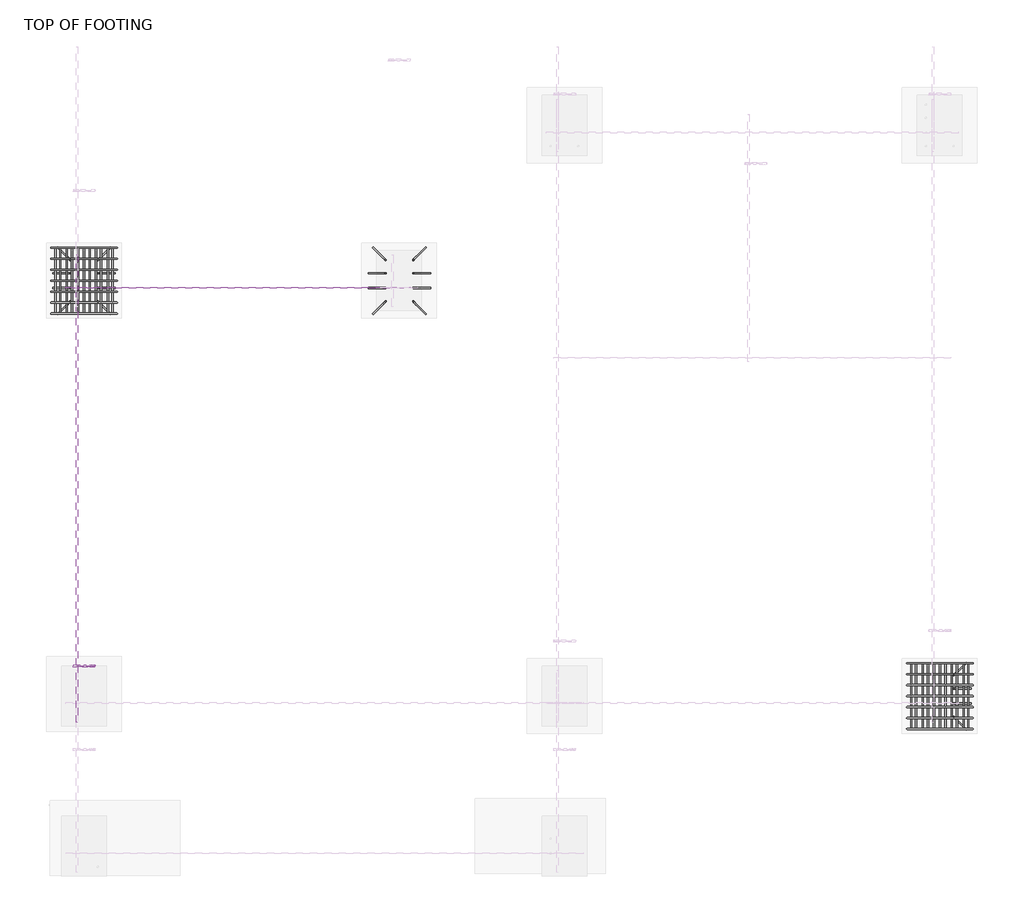
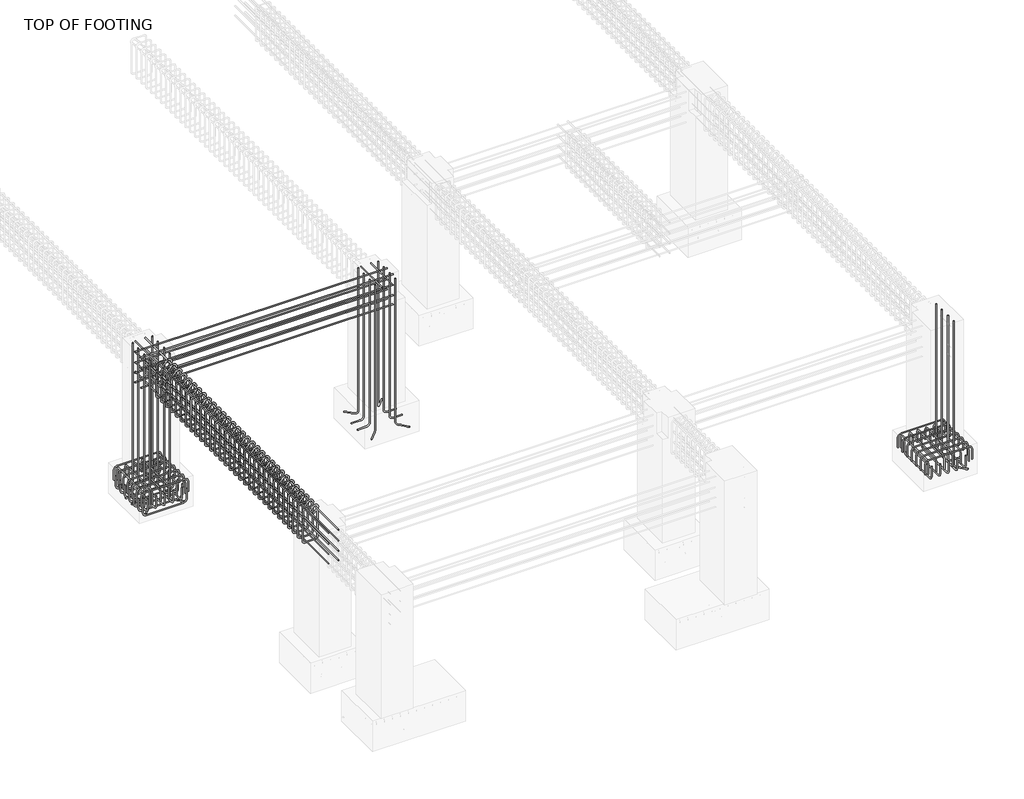
# One storey, part 4 of 8: 32 reinforcing bars.
"""IFC4 building model written with IfcOpenShell, lengths in millimetres."""

from ifc_helpers import new_model, si_unit, point, frame, origin, place, context, project, spatial, polyline, circle_curve, trimmed, segment, composite_curve, source, transform, mapped, element, save
from ifc_brep_helpers import swept_disk

model = new_model("IFC4")

# Units and contexts
model_context = context("Model", 3, world=origin())
ifc_project = project(units=[si_unit("LENGTHUNIT", "METRE", prefix="MILLI")], contexts=[model_context])

# Site, building, storey
site = spatial("IfcSite", under=ifc_project)
building = spatial("IfcBuilding", under=site)
storey = spatial("IfcBuildingStorey", under=building, Name="TOP OF FOOTING", Elevation=-1828.8)

# Reinforcing bars
placement = place(None, origin())
reinforcing_bar_shape = source(origin(), model_context, "Body", "SolidModel", [
    swept_disk(composite_curve([segment(polyline([(-6195.5877818, 3995.6420243, -2021.245224), (-6195.5877818, 3995.6420243, -2168.545224)]), True, "CONTINUOUS"), segment(trimmed(circle_curve(frame((-6241.9377818, 3995.6420243, -2168.545224), z_axis=(0.0, 1.0, 0.0), x_axis=(46.350000000000364, 0.0, 0.0)), 46.35), [point((-6195.5877818, 3995.6420243, -2168.545224))], [point((-6241.9377818, 3995.6420243, -2214.895224))], True, "CARTESIAN"), True, "CONTINUOUS"), segment(polyline([(-6241.9377818, 3995.6420243, -2214.895224), (-6762.8758647, 3995.6420243, -2214.895224)]), True, "CONTINUOUS"), segment(trimmed(circle_curve(frame((-6762.8758647, 3995.6420243, -2168.545224), z_axis=(0.0, 1.0, 0.0), x_axis=(0.0, 0.0, -46.34999999999991)), 46.35), [point((-6762.8758647, 3995.6420243, -2214.895224))], [point((-6809.2258647, 3995.6420243, -2168.545224))], True, "CARTESIAN"), True, "CONTINUOUS"), segment(polyline([(-6809.2258647, 3995.6420243, -2168.545224), (-6809.2258647, 3995.6420243, -2021.245224)]), True, "CONTINUOUS")], self_intersect=False), 6.35),
])
element("IfcReinforcingBar", 1, at=placement, inside=storey, context=model_context, shape_type="MappedRepresentation", body=[
    mapped(reinforcing_bar_shape, transform((0.0, 0.0, 0.0), x_axis=(1.0, 0.0, 0.0), y_axis=(0.0, 1.0, 0.0), z_axis=(0.0, 0.0, 1.0))),
    mapped(reinforcing_bar_shape, transform((0.0, -109.55, 0.0), x_axis=(1.0, 0.0, 0.0), y_axis=(0.0, 1.0, 0.0), z_axis=(0.0, 0.0, 1.0))),
    mapped(reinforcing_bar_shape, transform((0.0, -219.1, 0.0), x_axis=(1.0, 0.0, 0.0), y_axis=(0.0, 1.0, 0.0), z_axis=(0.0, 0.0, 1.0))),
    mapped(reinforcing_bar_shape, transform((0.0, -328.65, 0.0), x_axis=(1.0, 0.0, 0.0), y_axis=(0.0, 1.0, 0.0), z_axis=(0.0, 0.0, 1.0))),
    mapped(reinforcing_bar_shape, transform((0.0, -438.2, 0.0), x_axis=(1.0, 0.0, 0.0), y_axis=(0.0, 1.0, 0.0), z_axis=(0.0, 0.0, 1.0))),
    mapped(reinforcing_bar_shape, transform((0.0, -547.75, 0.0), x_axis=(1.0, 0.0, 0.0), y_axis=(0.0, 1.0, 0.0), z_axis=(0.0, 0.0, 1.0))),
    mapped(reinforcing_bar_shape, transform((0.0, -657.3, 0.0), x_axis=(1.0, 0.0, 0.0), y_axis=(0.0, 1.0, 0.0), z_axis=(0.0, 0.0, 1.0))),
])
reinforcing_bar_2_shape = source(origin(), model_context, "Body", "SolidModel", [
    swept_disk(composite_curve([segment(polyline([(-6831.1461367, 3995.6420243, -2068.8), (-6831.1461367, 3995.6420243, -1921.5)]), True, "CONTINUOUS"), segment(trimmed(circle_curve(frame((-6784.7961367, 3995.6420243, -1921.5), z_axis=(0.0, 1.0, 0.0), x_axis=(-46.350000000000364, 0.0, 0.0)), 46.35), [point((-6831.1461367, 3995.6420243, -1921.5))], [point((-6784.7961367, 3995.6420243, -1875.15))], True, "CARTESIAN"), True, "CONTINUOUS"), segment(polyline([(-6784.7961367, 3995.6420243, -1875.15), (-6220.1961367, 3995.6420243, -1875.15)]), True, "CONTINUOUS"), segment(trimmed(circle_curve(frame((-6220.1961367, 3995.6420243, -1921.5), z_axis=(0.0, 1.0, 0.0), x_axis=(0.0, 0.0, 46.34999999999991)), 46.35), [point((-6220.1961367, 3995.6420243, -1875.15))], [point((-6173.8461367, 3995.6420243, -1921.5))], True, "CARTESIAN"), True, "CONTINUOUS"), segment(polyline([(-6173.8461367, 3995.6420243, -1921.5), (-6173.8461367, 3995.6420243, -2068.8)]), True, "CONTINUOUS")], self_intersect=False), 6.35),
])
element("IfcReinforcingBar", 2, at=placement, inside=storey, context=model_context, shape_type="MappedRepresentation", body=[
    mapped(reinforcing_bar_2_shape, transform((0.0, 0.0, 0.0), x_axis=(1.0, 0.0, 0.0), y_axis=(0.0, 1.0, 0.0), z_axis=(0.0, 0.0, 1.0))),
    mapped(reinforcing_bar_2_shape, transform((0.0, -109.55, 0.0), x_axis=(1.0, 0.0, 0.0), y_axis=(0.0, 1.0, 0.0), z_axis=(0.0, 0.0, 1.0))),
    mapped(reinforcing_bar_2_shape, transform((0.0, -219.1, 0.0), x_axis=(1.0, 0.0, 0.0), y_axis=(0.0, 1.0, 0.0), z_axis=(0.0, 0.0, 1.0))),
    mapped(reinforcing_bar_2_shape, transform((0.0, -328.65, 0.0), x_axis=(1.0, 0.0, 0.0), y_axis=(0.0, 1.0, 0.0), z_axis=(0.0, 0.0, 1.0))),
    mapped(reinforcing_bar_2_shape, transform((0.0, -438.2, 0.0), x_axis=(1.0, 0.0, 0.0), y_axis=(0.0, 1.0, 0.0), z_axis=(0.0, 0.0, 1.0))),
    mapped(reinforcing_bar_2_shape, transform((0.0, -547.75, 0.0), x_axis=(1.0, 0.0, 0.0), y_axis=(0.0, 1.0, 0.0), z_axis=(0.0, 0.0, 1.0))),
    mapped(reinforcing_bar_2_shape, transform((0.0, -657.3, 0.0), x_axis=(1.0, 0.0, 0.0), y_axis=(0.0, 1.0, 0.0), z_axis=(0.0, 0.0, 1.0))),
])
reinforcing_bar_3_shape = source(origin(), model_context, "Body", "SolidModel", [
    swept_disk(composite_curve([segment(polyline([(-6219.0253093, 3995.6420243, -2080.9203068), (-6219.0253093, 3995.6420243, -1933.6203068)]), True, "CONTINUOUS"), segment(trimmed(circle_curve(frame((-6219.0253093, 3949.2920243, -1933.6203068), z_axis=(1.0, 0.0, 0.0), x_axis=(0.0, 46.34999999999991, 0.0)), 46.35), [point((-6219.0253093, 3995.6420243, -1933.6203068))], [point((-6219.0253093, 3949.2920243, -1887.2703068))], True, "CARTESIAN"), True, "CONTINUOUS"), segment(polyline([(-6219.0253093, 3949.2920243, -1887.2703068), (-6219.0253093, 3384.6920243, -1887.2703068)]), True, "CONTINUOUS"), segment(trimmed(circle_curve(frame((-6219.0253093, 3384.6920243, -1933.6203068), z_axis=(1.0, 0.0, 0.0), x_axis=(0.0, 0.0, 46.34999999999991)), 46.35), [point((-6219.0253093, 3384.6920243, -1887.2703068))], [point((-6219.0253093, 3338.3420243, -1933.6203068))], True, "CARTESIAN"), True, "CONTINUOUS"), segment(polyline([(-6219.0253093, 3338.3420243, -1933.6203068), (-6219.0253093, 3338.3420243, -2080.9203068)]), True, "CONTINUOUS")], self_intersect=False), 6.35),
])
element("IfcReinforcingBar", 3, at=placement, inside=storey, context=model_context, shape_type="MappedRepresentation", body=[
    mapped(reinforcing_bar_3_shape, transform((0.0, 0.0, 0.0), x_axis=(1.0, 0.0, 0.0), y_axis=(0.0, 1.0, 0.0), z_axis=(0.0, 0.0, 1.0))),
    mapped(reinforcing_bar_3_shape, transform((-113.9683653, 0.0, 0.0), x_axis=(1.0, 0.0, 0.0), y_axis=(0.0, 1.0, 0.0), z_axis=(0.0, 0.0, 1.0))),
    mapped(reinforcing_bar_3_shape, transform((-227.9367307, 0.0, 0.0), x_axis=(1.0, 0.0, 0.0), y_axis=(0.0, 1.0, 0.0), z_axis=(0.0, 0.0, 1.0))),
    mapped(reinforcing_bar_3_shape, transform((-341.905096, 0.0, 0.0), x_axis=(1.0, 0.0, 0.0), y_axis=(0.0, 1.0, 0.0), z_axis=(0.0, 0.0, 1.0))),
    mapped(reinforcing_bar_3_shape, transform((-455.8734613, 0.0, 0.0), x_axis=(1.0, 0.0, 0.0), y_axis=(0.0, 1.0, 0.0), z_axis=(0.0, 0.0, 1.0))),
    mapped(reinforcing_bar_3_shape, transform((-569.8418267, 0.0, 0.0), x_axis=(1.0, 0.0, 0.0), y_axis=(0.0, 1.0, 0.0), z_axis=(0.0, 0.0, 1.0))),
])
reinforcing_bar_4_shape = source(origin(), model_context, "Body", "SolidModel", [
    swept_disk(composite_curve([segment(polyline([(-6741.3656272, 3995.6420243, -1984.9681267), (-6741.3656272, 3995.6420243, -2132.2681267)]), True, "CONTINUOUS"), segment(trimmed(circle_curve(frame((-6741.3656272, 3949.2920243, -2132.2681267), z_axis=(-1.0, 0.0, 0.0), x_axis=(0.0, 46.34999999999991, 0.0)), 46.35), [point((-6741.3656272, 3995.6420243, -2132.2681267))], [point((-6741.3656272, 3949.2920243, -2178.6181267))], True, "CARTESIAN"), True, "CONTINUOUS"), segment(polyline([(-6741.3656272, 3949.2920243, -2178.6181267), (-6741.3656272, 3384.6920243, -2178.6181267)]), True, "CONTINUOUS"), segment(trimmed(circle_curve(frame((-6741.3656272, 3384.6920243, -2132.2681267), z_axis=(-1.0, 0.0, 0.0), x_axis=(0.0, 0.0, -46.350000000000364)), 46.35), [point((-6741.3656272, 3384.6920243, -2178.6181267))], [point((-6741.3656272, 3338.3420243, -2132.2681267))], True, "CARTESIAN"), True, "CONTINUOUS"), segment(polyline([(-6741.3656272, 3338.3420243, -2132.2681267), (-6741.3656272, 3338.3420243, -1984.9681267)]), True, "CONTINUOUS")], self_intersect=False), 6.35),
])
element("IfcReinforcingBar", 4, at=placement, inside=storey, context=model_context, shape_type="MappedRepresentation", body=[
    mapped(reinforcing_bar_4_shape, transform((0.0, 0.0, 0.0), x_axis=(1.0, 0.0, 0.0), y_axis=(0.0, 1.0, 0.0), z_axis=(0.0, 0.0, 1.0))),
    mapped(reinforcing_bar_4_shape, transform((119.2770606, 0.0, 0.0), x_axis=(1.0, 0.0, 0.0), y_axis=(0.0, 1.0, 0.0), z_axis=(0.0, 0.0, 1.0))),
    mapped(reinforcing_bar_4_shape, transform((238.5541211, 0.0, 0.0), x_axis=(1.0, 0.0, 0.0), y_axis=(0.0, 1.0, 0.0), z_axis=(0.0, 0.0, 1.0))),
    mapped(reinforcing_bar_4_shape, transform((357.8311817, 0.0, 0.0), x_axis=(1.0, 0.0, 0.0), y_axis=(0.0, 1.0, 0.0), z_axis=(0.0, 0.0, 1.0))),
    mapped(reinforcing_bar_4_shape, transform((477.1082423, 0.0, 0.0), x_axis=(1.0, 0.0, 0.0), y_axis=(0.0, 1.0, 0.0), z_axis=(0.0, 0.0, 1.0))),
])
reinforcing_bar_5_shape = source(origin(), model_context, "Body", "SolidModel", [
    swept_disk(composite_curve([segment(polyline([(1718.8538633, -154.3579757, -2068.8), (1718.8538633, -154.3579757, -1921.5)]), True, "CONTINUOUS"), segment(trimmed(circle_curve(frame((1765.2038633, -154.3579757, -1921.5), z_axis=(0.0, 1.0, 0.0), x_axis=(-46.34999999999991, 0.0, 0.0)), 46.35), [point((1718.8538633, -154.3579757, -1921.5))], [point((1765.2038633, -154.3579757, -1875.15))], True, "CARTESIAN"), True, "CONTINUOUS"), segment(polyline([(1765.2038633, -154.3579757, -1875.15), (2329.8038633, -154.3579757, -1875.15)]), True, "CONTINUOUS"), segment(trimmed(circle_curve(frame((2329.8038633, -154.3579757, -1921.5), z_axis=(0.0, 1.0, 0.0), x_axis=(0.0, 0.0, 46.34999999999991)), 46.35), [point((2329.8038633, -154.3579757, -1875.15))], [point((2376.1538633, -154.3579757, -1921.5))], True, "CARTESIAN"), True, "CONTINUOUS"), segment(polyline([(2376.1538633, -154.3579757, -1921.5), (2376.1538633, -154.3579757, -2068.8)]), True, "CONTINUOUS")], self_intersect=False), 6.35),
])
element("IfcReinforcingBar", 5, at=placement, inside=storey, context=model_context, shape_type="MappedRepresentation", body=[
    mapped(reinforcing_bar_5_shape, transform((0.0, 0.0, 0.0), x_axis=(1.0, 0.0, 0.0), y_axis=(0.0, 1.0, 0.0), z_axis=(0.0, 0.0, 1.0))),
    mapped(reinforcing_bar_5_shape, transform((0.0, -109.55, 0.0), x_axis=(1.0, 0.0, 0.0), y_axis=(0.0, 1.0, 0.0), z_axis=(0.0, 0.0, 1.0))),
    mapped(reinforcing_bar_5_shape, transform((0.0, -219.1, 0.0), x_axis=(1.0, 0.0, 0.0), y_axis=(0.0, 1.0, 0.0), z_axis=(0.0, 0.0, 1.0))),
    mapped(reinforcing_bar_5_shape, transform((0.0, -328.65, 0.0), x_axis=(1.0, 0.0, 0.0), y_axis=(0.0, 1.0, 0.0), z_axis=(0.0, 0.0, 1.0))),
    mapped(reinforcing_bar_5_shape, transform((0.0, -438.2, 0.0), x_axis=(1.0, 0.0, 0.0), y_axis=(0.0, 1.0, 0.0), z_axis=(0.0, 0.0, 1.0))),
    mapped(reinforcing_bar_5_shape, transform((0.0, -547.75, 0.0), x_axis=(1.0, 0.0, 0.0), y_axis=(0.0, 1.0, 0.0), z_axis=(0.0, 0.0, 1.0))),
    mapped(reinforcing_bar_5_shape, transform((0.0, -657.3, 0.0), x_axis=(1.0, 0.0, 0.0), y_axis=(0.0, 1.0, 0.0), z_axis=(0.0, 0.0, 1.0))),
])
reinforcing_bar_6_shape = source(origin(), model_context, "Body", "SolidModel", [
    swept_disk(composite_curve([segment(polyline([(2330.9746907, -154.3579757, -2080.9203068), (2330.9746907, -154.3579757, -1933.6203068)]), True, "CONTINUOUS"), segment(trimmed(circle_curve(frame((2330.9746907, -200.7079757, -1933.6203068), z_axis=(1.0, 0.0, 0.0), x_axis=(0.0, 46.349999999999994, 0.0)), 46.35), [point((2330.9746907, -154.3579757, -1933.6203068))], [point((2330.9746907, -200.7079757, -1887.2703068))], True, "CARTESIAN"), True, "CONTINUOUS"), segment(polyline([(2330.9746907, -200.7079757, -1887.2703068), (2330.9746907, -765.3079757, -1887.2703068)]), True, "CONTINUOUS"), segment(trimmed(circle_curve(frame((2330.9746907, -765.3079757, -1933.6203068), z_axis=(1.0, 0.0, 0.0), x_axis=(0.0, 0.0, 46.34999999999991)), 46.35), [point((2330.9746907, -765.3079757, -1887.2703068))], [point((2330.9746907, -811.6579757, -1933.6203068))], True, "CARTESIAN"), True, "CONTINUOUS"), segment(polyline([(2330.9746907, -811.6579757, -1933.6203068), (2330.9746907, -811.6579757, -2080.9203068)]), True, "CONTINUOUS")], self_intersect=False), 6.35),
])
element("IfcReinforcingBar", 6, at=placement, inside=storey, context=model_context, shape_type="MappedRepresentation", body=[
    mapped(reinforcing_bar_6_shape, transform((0.0, 0.0, 0.0), x_axis=(1.0, 0.0, 0.0), y_axis=(0.0, 1.0, 0.0), z_axis=(0.0, 0.0, 1.0))),
    mapped(reinforcing_bar_6_shape, transform((-113.9683653, 0.0, 0.0), x_axis=(1.0, 0.0, 0.0), y_axis=(0.0, 1.0, 0.0), z_axis=(0.0, 0.0, 1.0))),
    mapped(reinforcing_bar_6_shape, transform((-227.9367307, 0.0, 0.0), x_axis=(1.0, 0.0, 0.0), y_axis=(0.0, 1.0, 0.0), z_axis=(0.0, 0.0, 1.0))),
    mapped(reinforcing_bar_6_shape, transform((-341.905096, 0.0, 0.0), x_axis=(1.0, 0.0, 0.0), y_axis=(0.0, 1.0, 0.0), z_axis=(0.0, 0.0, 1.0))),
    mapped(reinforcing_bar_6_shape, transform((-455.8734613, 0.0, 0.0), x_axis=(1.0, 0.0, 0.0), y_axis=(0.0, 1.0, 0.0), z_axis=(0.0, 0.0, 1.0))),
    mapped(reinforcing_bar_6_shape, transform((-569.8418267, 0.0, 0.0), x_axis=(1.0, 0.0, 0.0), y_axis=(0.0, 1.0, 0.0), z_axis=(0.0, 0.0, 1.0))),
])
reinforcing_bar_7_shape = source(origin(), model_context, "Body", "SolidModel", [
    swept_disk(composite_curve([segment(polyline([(1808.6343728, -154.3579757, -1984.9681267), (1808.6343728, -154.3579757, -2132.2681267)]), True, "CONTINUOUS"), segment(trimmed(circle_curve(frame((1808.6343728, -200.7079757, -2132.2681267), z_axis=(-1.0, 0.0, 0.0), x_axis=(0.0, 46.349999999999994, 0.0)), 46.35), [point((1808.6343728, -154.3579757, -2132.2681267))], [point((1808.6343728, -200.7079757, -2178.6181267))], True, "CARTESIAN"), True, "CONTINUOUS"), segment(polyline([(1808.6343728, -200.7079757, -2178.6181267), (1808.6343728, -765.3079757, -2178.6181267)]), True, "CONTINUOUS"), segment(trimmed(circle_curve(frame((1808.6343728, -765.3079757, -2132.2681267), z_axis=(-1.0, 0.0, 0.0), x_axis=(0.0, 0.0, -46.350000000000364)), 46.35), [point((1808.6343728, -765.3079757, -2178.6181267))], [point((1808.6343728, -811.6579757, -2132.2681267))], True, "CARTESIAN"), True, "CONTINUOUS"), segment(polyline([(1808.6343728, -811.6579757, -2132.2681267), (1808.6343728, -811.6579757, -1984.9681267)]), True, "CONTINUOUS")], self_intersect=False), 6.35),
])
element("IfcReinforcingBar", 7, at=placement, inside=storey, context=model_context, shape_type="MappedRepresentation", body=[
    mapped(reinforcing_bar_7_shape, transform((0.0, 0.0, 0.0), x_axis=(1.0, 0.0, 0.0), y_axis=(0.0, 1.0, 0.0), z_axis=(0.0, 0.0, 1.0))),
    mapped(reinforcing_bar_7_shape, transform((119.2770606, 0.0, 0.0), x_axis=(1.0, 0.0, 0.0), y_axis=(0.0, 1.0, 0.0), z_axis=(0.0, 0.0, 1.0))),
    mapped(reinforcing_bar_7_shape, transform((238.5541211, 0.0, 0.0), x_axis=(1.0, 0.0, 0.0), y_axis=(0.0, 1.0, 0.0), z_axis=(0.0, 0.0, 1.0))),
    mapped(reinforcing_bar_7_shape, transform((357.8311817, 0.0, 0.0), x_axis=(1.0, 0.0, 0.0), y_axis=(0.0, 1.0, 0.0), z_axis=(0.0, 0.0, 1.0))),
    mapped(reinforcing_bar_7_shape, transform((477.1082423, 0.0, 0.0), x_axis=(1.0, 0.0, 0.0), y_axis=(0.0, 1.0, 0.0), z_axis=(0.0, 0.0, 1.0))),
])
reinforcing_bar_8_shape = source(origin(), model_context, "Body", "SolidModel", [
    swept_disk(composite_curve([segment(polyline([(-6815.4438347, 3742.1344308, -2192.6897268), (-6687.1151723, 3742.1344308, -2192.6897268)]), True, "CONTINUOUS"), segment(trimmed(circle_curve(frame((-6687.1151723, 3742.1344308, -2146.3397268), z_axis=(0.0, -1.0, 0.0), x_axis=(0.0, 0.0, -46.34999999999991)), 46.35), [point((-6687.1151723, 3742.1344308, -2192.6897268))], [point((-6640.7651723, 3742.1344308, -2146.3397268))], True, "CARTESIAN"), True, "CONTINUOUS"), segment(polyline([(-6640.7651723, 3742.1344308, -2146.3397268), (-6640.7651723, 3742.1344308, -40.0)]), True, "CONTINUOUS")], self_intersect=False), 6.35),
])
element("IfcReinforcingBar", 8, at=placement, inside=storey, context=model_context, shape_type="MappedRepresentation", body=[
    mapped(reinforcing_bar_8_shape, transform((0.0, 0.0, 0.0), x_axis=(1.0, 0.0, 0.0), y_axis=(0.0, 1.0, 0.0), z_axis=(0.0, 0.0, 1.0))),
    mapped(reinforcing_bar_8_shape, transform((0.0, -147.7903727, 0.0), x_axis=(1.0, 0.0, 0.0), y_axis=(0.0, 1.0, 0.0), z_axis=(0.0, 0.0, 1.0))),
])
element("IfcReinforcingBar", 9, at=placement, inside=storey, context=model_context, shape_type="SolidModel", body=[
    swept_disk(composite_curve([segment(polyline([(-6768.0144002, 3332.6300935, -2192.6897268), (-6673.5395717, 3427.1049221, -2192.6897268)]), True, "CONTINUOUS"), segment(trimmed(circle_curve(frame((-6673.5395717, 3427.1049221, -2146.3397268), z_axis=(0.7071067811865476, -0.7071067811865475, 0.0), x_axis=(0.0, 0.0, -46.34999999999991)), 46.35), [point((-6673.5395717, 3427.1049221, -2192.6897268))], [point((-6640.7651723, 3459.8793214, -2146.3397268))], True, "CARTESIAN"), True, "CONTINUOUS"), segment(polyline([(-6640.7651723, 3459.8793214, -2146.3397268), (-6640.7651723, 3459.8793214, -40.0)]), True, "CONTINUOUS")], self_intersect=False), 6.35),
])
element("IfcReinforcingBar", 10, at=placement, inside=storey, context=model_context, shape_type="SolidModel", body=[
    swept_disk(composite_curve([segment(polyline([(-6236.9778732, 3332.6300935, -2192.6897268), (-6331.4527018, 3427.1049221, -2192.6897268)]), True, "CONTINUOUS"), segment(trimmed(circle_curve(frame((-6331.4527018, 3427.1049221, -2146.3397268), z_axis=(0.7071067811865753, 0.7071067811865197, 0.0), x_axis=(0.0, 0.0, -46.34999999999991)), 46.35), [point((-6331.4527018, 3427.1049221, -2192.6897268))], [point((-6364.2271011, 3459.8793214, -2146.3397268))], True, "CARTESIAN"), True, "CONTINUOUS"), segment(polyline([(-6364.2271011, 3459.8793214, -2146.3397268), (-6364.2271011, 3459.8793214, -40.0)]), True, "CONTINUOUS")], self_intersect=False), 6.35),
])
element("IfcReinforcingBar", 11, at=placement, inside=storey, context=model_context, shape_type="SolidModel", body=[
    swept_disk(composite_curve([segment(polyline([(-6768.0144002, 4001.353955, -2192.6897268), (-6673.5395717, 3906.8791264, -2192.6897268)]), True, "CONTINUOUS"), segment(trimmed(circle_curve(frame((-6673.5395717, 3906.8791264, -2146.3397268), z_axis=(-0.7071067811865389, -0.7071067811865561, 0.0), x_axis=(0.0, 0.0, -46.34999999999991)), 46.35), [point((-6673.5395717, 3906.8791264, -2192.6897268))], [point((-6640.7651723, 3874.1047271, -2146.3397268))], True, "CARTESIAN"), True, "CONTINUOUS"), segment(polyline([(-6640.7651723, 3874.1047271, -2146.3397268), (-6640.7651723, 3874.1047271, -40.0)]), True, "CONTINUOUS")], self_intersect=False), 6.35),
])
element("IfcReinforcingBar", 12, at=placement, inside=storey, context=model_context, shape_type="SolidModel", body=[
    swept_disk(composite_curve([segment(polyline([(-6236.9778732, 4001.353955, -2192.6897268), (-6331.4527018, 3906.8791264, -2192.6897268)]), True, "CONTINUOUS"), segment(trimmed(circle_curve(frame((-6331.4527018, 3906.8791264, -2146.3397268), z_axis=(-0.707106781186584, 0.707106781186511, 0.0), x_axis=(0.0, 0.0, -46.34999999999991)), 46.35), [point((-6331.4527018, 3906.8791264, -2192.6897268))], [point((-6364.2271011, 3874.1047271, -2146.3397268))], True, "CARTESIAN"), True, "CONTINUOUS"), segment(polyline([(-6364.2271011, 3874.1047271, -2146.3397268), (-6364.2271011, 3874.1047271, -40.0)]), True, "CONTINUOUS")], self_intersect=False), 6.35),
])
reinforcing_bar_9_shape = source(origin(), model_context, "Body", "SolidModel", [
    swept_disk(composite_curve([segment(polyline([(-6189.5484388, 3742.1344308, -2192.6897268), (-6317.8771011, 3742.1344308, -2192.6897268)]), True, "CONTINUOUS"), segment(trimmed(circle_curve(frame((-6317.8771011, 3742.1344308, -2146.3397268), z_axis=(0.0, 1.0, 0.0), x_axis=(0.0, 0.0, -46.34999999999991)), 46.35), [point((-6317.8771011, 3742.1344308, -2192.6897268))], [point((-6364.2271011, 3742.1344308, -2146.3397268))], True, "CARTESIAN"), True, "CONTINUOUS"), segment(polyline([(-6364.2271011, 3742.1344308, -2146.3397268), (-6364.2271011, 3742.1344308, -40.0)]), True, "CONTINUOUS")], self_intersect=False), 6.35),
])
element("IfcReinforcingBar", 13, at=placement, inside=storey, context=model_context, shape_type="MappedRepresentation", body=[
    mapped(reinforcing_bar_9_shape, transform((0.0, 0.0, 0.0), x_axis=(1.0, 0.0, 0.0), y_axis=(0.0, 1.0, 0.0), z_axis=(0.0, 0.0, 1.0))),
    mapped(reinforcing_bar_9_shape, transform((0.0, -147.7903727, 0.0), x_axis=(1.0, 0.0, 0.0), y_axis=(0.0, 1.0, 0.0), z_axis=(0.0, 0.0, 1.0))),
])
element("IfcReinforcingBar", 14, at=placement, inside=storey, context=model_context, shape_type="SolidModel", body=[
    swept_disk(composite_curve([segment(polyline([(2313.0221268, -817.3699065, -2192.6897268), (2218.5472982, -722.8950779, -2192.6897268)]), True, "CONTINUOUS"), segment(trimmed(circle_curve(frame((2218.5472982, -722.8950779, -2146.3397268), z_axis=(0.7071067811865753, 0.7071067811865197, 0.0), x_axis=(0.0, 0.0, -46.34999999999991)), 46.35), [point((2218.5472982, -722.8950779, -2192.6897268))], [point((2185.7728989, -690.1206786, -2146.3397268))], True, "CARTESIAN"), True, "CONTINUOUS"), segment(polyline([(2185.7728989, -690.1206786, -2146.3397268), (2185.7728989, -690.1206786, -40.0)]), True, "CONTINUOUS")], self_intersect=False), 6.35),
])
element("IfcReinforcingBar", 15, at=placement, inside=storey, context=model_context, shape_type="SolidModel", body=[
    swept_disk(composite_curve([segment(polyline([(2313.0221268, -148.646045, -2192.6897268), (2218.5472982, -243.1208736, -2192.6897268)]), True, "CONTINUOUS"), segment(trimmed(circle_curve(frame((2218.5472982, -243.1208736, -2146.3397268), z_axis=(-0.707106781186584, 0.707106781186511, 0.0), x_axis=(0.0, 0.0, -46.34999999999991)), 46.35), [point((2218.5472982, -243.1208736, -2192.6897268))], [point((2185.7728989, -275.8952729, -2146.3397268))], True, "CARTESIAN"), True, "CONTINUOUS"), segment(polyline([(2185.7728989, -275.8952729, -2146.3397268), (2185.7728989, -275.8952729, -40.0)]), True, "CONTINUOUS")], self_intersect=False), 6.35),
])
reinforcing_bar_10_shape = source(origin(), model_context, "Body", "SolidModel", [
    swept_disk(composite_curve([segment(polyline([(2360.4515612, -407.8655692, -2192.6897268), (2232.1228989, -407.8655692, -2192.6897268)]), True, "CONTINUOUS"), segment(trimmed(circle_curve(frame((2232.1228989, -407.8655692, -2146.3397268), z_axis=(0.0, 1.0, 0.0), x_axis=(0.0, 0.0, -46.34999999999991)), 46.35), [point((2232.1228989, -407.8655692, -2192.6897268))], [point((2185.7728989, -407.8655692, -2146.3397268))], True, "CARTESIAN"), True, "CONTINUOUS"), segment(polyline([(2185.7728989, -407.8655692, -2146.3397268), (2185.7728989, -407.8655692, -40.0)]), True, "CONTINUOUS")], self_intersect=False), 6.35),
])
element("IfcReinforcingBar", 16, at=placement, inside=storey, context=model_context, shape_type="MappedRepresentation", body=[
    mapped(reinforcing_bar_10_shape, transform((0.0, 0.0, 0.0), x_axis=(1.0, 0.0, 0.0), y_axis=(0.0, 1.0, 0.0), z_axis=(0.0, 0.0, 1.0))),
    mapped(reinforcing_bar_10_shape, transform((0.0, -147.7903727, 0.0), x_axis=(1.0, 0.0, 0.0), y_axis=(0.0, 1.0, 0.0), z_axis=(0.0, 0.0, 1.0))),
])
reinforcing_bar_11_shape = source(origin(), model_context, "Body", "SolidModel", [
    swept_disk(composite_curve([segment(polyline([(-3665.4438347, 3742.1344308, -2192.6897268), (-3537.1151723, 3742.1344308, -2192.6897268)]), True, "CONTINUOUS"), segment(trimmed(circle_curve(frame((-3537.1151723, 3742.1344308, -2146.3397268), z_axis=(0.0, -1.0, 0.0), x_axis=(0.0, 0.0, -46.34999999999991)), 46.35), [point((-3537.1151723, 3742.1344308, -2192.6897268))], [point((-3490.7651723, 3742.1344308, -2146.3397268))], True, "CARTESIAN"), True, "CONTINUOUS"), segment(polyline([(-3490.7651723, 3742.1344308, -2146.3397268), (-3490.7651723, 3742.1344308, -40.0)]), True, "CONTINUOUS")], self_intersect=False), 6.35),
])
element("IfcReinforcingBar", 17, at=placement, inside=storey, context=model_context, shape_type="MappedRepresentation", body=[
    mapped(reinforcing_bar_11_shape, transform((0.0, 0.0, 0.0), x_axis=(1.0, 0.0, 0.0), y_axis=(0.0, 1.0, 0.0), z_axis=(0.0, 0.0, 1.0))),
    mapped(reinforcing_bar_11_shape, transform((0.0, -147.7903727, 0.0), x_axis=(1.0, 0.0, 0.0), y_axis=(0.0, 1.0, 0.0), z_axis=(0.0, 0.0, 1.0))),
])
element("IfcReinforcingBar", 18, at=placement, inside=storey, context=model_context, shape_type="SolidModel", body=[
    swept_disk(composite_curve([segment(polyline([(-3618.0144002, 3332.6300935, -2192.6897268), (-3523.5395717, 3427.1049221, -2192.6897268)]), True, "CONTINUOUS"), segment(trimmed(circle_curve(frame((-3523.5395717, 3427.1049221, -2146.3397268), z_axis=(0.7071067811865476, -0.7071067811865475, 0.0), x_axis=(0.0, 0.0, -46.34999999999991)), 46.35), [point((-3523.5395717, 3427.1049221, -2192.6897268))], [point((-3490.7651723, 3459.8793214, -2146.3397268))], True, "CARTESIAN"), True, "CONTINUOUS"), segment(polyline([(-3490.7651723, 3459.8793214, -2146.3397268), (-3490.7651723, 3459.8793214, -40.0)]), True, "CONTINUOUS")], self_intersect=False), 6.35),
])
element("IfcReinforcingBar", 19, at=placement, inside=storey, context=model_context, shape_type="SolidModel", body=[
    swept_disk(composite_curve([segment(polyline([(-3086.9778732, 3332.6300935, -2192.6897268), (-3181.4527018, 3427.1049221, -2192.6897268)]), True, "CONTINUOUS"), segment(trimmed(circle_curve(frame((-3181.4527018, 3427.1049221, -2146.3397268), z_axis=(0.7071067811865753, 0.7071067811865197, 0.0), x_axis=(0.0, 0.0, -46.34999999999991)), 46.35), [point((-3181.4527018, 3427.1049221, -2192.6897268))], [point((-3214.2271011, 3459.8793214, -2146.3397268))], True, "CARTESIAN"), True, "CONTINUOUS"), segment(polyline([(-3214.2271011, 3459.8793214, -2146.3397268), (-3214.2271011, 3459.8793214, -40.0)]), True, "CONTINUOUS")], self_intersect=False), 6.35),
])
element("IfcReinforcingBar", 20, at=placement, inside=storey, context=model_context, shape_type="SolidModel", body=[
    swept_disk(composite_curve([segment(polyline([(-3618.0144002, 4001.353955, -2192.6897268), (-3523.5395717, 3906.8791264, -2192.6897268)]), True, "CONTINUOUS"), segment(trimmed(circle_curve(frame((-3523.5395717, 3906.8791264, -2146.3397268), z_axis=(-0.7071067811865389, -0.7071067811865561, 0.0), x_axis=(0.0, 0.0, -46.34999999999991)), 46.35), [point((-3523.5395717, 3906.8791264, -2192.6897268))], [point((-3490.7651723, 3874.1047271, -2146.3397268))], True, "CARTESIAN"), True, "CONTINUOUS"), segment(polyline([(-3490.7651723, 3874.1047271, -2146.3397268), (-3490.7651723, 3874.1047271, -40.0)]), True, "CONTINUOUS")], self_intersect=False), 6.35),
])
element("IfcReinforcingBar", 21, at=placement, inside=storey, context=model_context, shape_type="SolidModel", body=[
    swept_disk(composite_curve([segment(polyline([(-3086.9778732, 4001.353955, -2192.6897268), (-3181.4527018, 3906.8791264, -2192.6897268)]), True, "CONTINUOUS"), segment(trimmed(circle_curve(frame((-3181.4527018, 3906.8791264, -2146.3397268), z_axis=(-0.707106781186584, 0.707106781186511, 0.0), x_axis=(0.0, 0.0, -46.34999999999991)), 46.35), [point((-3181.4527018, 3906.8791264, -2192.6897268))], [point((-3214.2271011, 3874.1047271, -2146.3397268))], True, "CARTESIAN"), True, "CONTINUOUS"), segment(polyline([(-3214.2271011, 3874.1047271, -2146.3397268), (-3214.2271011, 3874.1047271, -40.0)]), True, "CONTINUOUS")], self_intersect=False), 6.35),
])
reinforcing_bar_12_shape = source(origin(), model_context, "Body", "SolidModel", [
    swept_disk(composite_curve([segment(polyline([(-3039.5484388, 3742.1344308, -2192.6897268), (-3167.8771011, 3742.1344308, -2192.6897268)]), True, "CONTINUOUS"), segment(trimmed(circle_curve(frame((-3167.8771011, 3742.1344308, -2146.3397268), z_axis=(0.0, 1.0, 0.0), x_axis=(0.0, 0.0, -46.34999999999991)), 46.35), [point((-3167.8771011, 3742.1344308, -2192.6897268))], [point((-3214.2271011, 3742.1344308, -2146.3397268))], True, "CARTESIAN"), True, "CONTINUOUS"), segment(polyline([(-3214.2271011, 3742.1344308, -2146.3397268), (-3214.2271011, 3742.1344308, -40.0)]), True, "CONTINUOUS")], self_intersect=False), 6.35),
])
element("IfcReinforcingBar", 22, at=placement, inside=storey, context=model_context, shape_type="MappedRepresentation", body=[
    mapped(reinforcing_bar_12_shape, transform((0.0, 0.0, 0.0), x_axis=(1.0, 0.0, 0.0), y_axis=(0.0, 1.0, 0.0), z_axis=(0.0, 0.0, 1.0))),
    mapped(reinforcing_bar_12_shape, transform((0.0, -147.7903727, 0.0), x_axis=(1.0, 0.0, 0.0), y_axis=(0.0, 1.0, 0.0), z_axis=(0.0, 0.0, 1.0))),
])
reinforcing_bar_13_shape = source(origin(), model_context, "Body", "SolidModel", [
    swept_disk(composite_curve([segment(polyline([(-6508.1074973, -176.6579757, -111.2757654), (-6452.3639343, -176.6579757, -55.5322024)]), True, "CONTINUOUS"), segment(trimmed(circle_curve(frame((-6430.1961367, -176.6579757, -77.7), z_axis=(0.0, 1.0, 0.0), x_axis=(-22.167797600000085, 0.0, 22.1677976)), 31.35), [point((-6452.3639343, -176.6579757, -55.5322024))], [point((-6398.8461367, -176.6579757, -77.7))], True, "CARTESIAN"), True, "CONTINUOUS"), segment(polyline([(-6398.8461367, -176.6579757, -77.7), (-6398.8461367, -176.6579757, -522.3)]), True, "CONTINUOUS"), segment(trimmed(circle_curve(frame((-6430.1961367, -176.6579757, -522.3), z_axis=(0.0, 1.0, 0.0), x_axis=(31.350000000000364, 0.0, 0.0)), 31.35), [point((-6398.8461367, -176.6579757, -522.3))], [point((-6430.1961367, -176.6579757, -553.65))], True, "CARTESIAN"), True, "CONTINUOUS"), segment(polyline([(-6430.1961367, -176.6579757, -553.65), (-6574.7961367, -176.6579757, -553.65)]), True, "CONTINUOUS"), segment(trimmed(circle_curve(frame((-6574.7961367, -177.4425614, -522.3098193), z_axis=(0.0, 0.9996867842138424, 0.025026655153786322), x_axis=(0.0, 0.7845856999999796, -31.34018070000002)), 31.35), [point((-6574.7961367, -176.6579757, -553.65))], [point((-6606.1461367, -177.4425614, -522.3098193))], True, "CARTESIAN"), True, "CONTINUOUS"), segment(polyline([(-6606.1461367, -177.4425614, -522.3098193), (-6606.1461367, -188.5733901, -77.6901807)]), True, "CONTINUOUS"), segment(trimmed(circle_curve(frame((-6574.7961367, -188.5733901, -77.6901807), z_axis=(0.0, 0.9996867842138424, 0.025026655153786322), x_axis=(-31.350000000000364, 0.0, 0.0)), 31.35), [point((-6606.1461367, -188.5733901, -77.6901807))], [point((-6574.7961367, -189.3579757, -46.35))], True, "CARTESIAN"), True, "CONTINUOUS"), segment(polyline([(-6574.7961367, -189.3579757, -46.35), (-6430.1961367, -189.3579757, -46.35)]), True, "CONTINUOUS"), segment(trimmed(circle_curve(frame((-6430.1961367, -189.3579757, -77.7), z_axis=(0.0, 1.0, 0.0), x_axis=(0.0, 0.0, 31.35)), 31.35), [point((-6430.1961367, -189.3579757, -46.35))], [point((-6408.0283391, -189.3579757, -99.8677976))], True, "CARTESIAN"), True, "CONTINUOUS"), segment(polyline([(-6408.0283391, -189.3579757, -99.8677976), (-6463.7719021, -189.3579757, -155.6113605)]), True, "CONTINUOUS")], self_intersect=False), 6.35),
])
element("IfcReinforcingBar", 23, at=placement, inside=storey, context=model_context, shape_type="MappedRepresentation", body=[
    mapped(reinforcing_bar_13_shape, transform((0.0, 0.0, 0.0), x_axis=(1.0, 0.0, 0.0), y_axis=(0.0, 1.0, 0.0), z_axis=(0.0, 0.0, 1.0))),
    mapped(reinforcing_bar_13_shape, transform((0.0, 117.91, 0.0), x_axis=(1.0, 0.0, 0.0), y_axis=(0.0, 1.0, 0.0), z_axis=(0.0, 0.0, 1.0))),
    mapped(reinforcing_bar_13_shape, transform((0.0, 235.82, 0.0), x_axis=(1.0, 0.0, 0.0), y_axis=(0.0, 1.0, 0.0), z_axis=(0.0, 0.0, 1.0))),
    mapped(reinforcing_bar_13_shape, transform((0.0, 353.73, 0.0), x_axis=(1.0, 0.0, 0.0), y_axis=(0.0, 1.0, 0.0), z_axis=(0.0, 0.0, 1.0))),
    mapped(reinforcing_bar_13_shape, transform((0.0, 471.64, 0.0), x_axis=(1.0, 0.0, 0.0), y_axis=(0.0, 1.0, 0.0), z_axis=(0.0, 0.0, 1.0))),
    mapped(reinforcing_bar_13_shape, transform((0.0, 589.55, 0.0), x_axis=(1.0, 0.0, 0.0), y_axis=(0.0, 1.0, 0.0), z_axis=(0.0, 0.0, 1.0))),
    mapped(reinforcing_bar_13_shape, transform((0.0, 707.46, 0.0), x_axis=(1.0, 0.0, 0.0), y_axis=(0.0, 1.0, 0.0), z_axis=(0.0, 0.0, 1.0))),
    mapped(reinforcing_bar_13_shape, transform((0.0, 825.37, 0.0), x_axis=(1.0, 0.0, 0.0), y_axis=(0.0, 1.0, 0.0), z_axis=(0.0, 0.0, 1.0))),
    mapped(reinforcing_bar_13_shape, transform((0.0, 943.28, 0.0), x_axis=(1.0, 0.0, 0.0), y_axis=(0.0, 1.0, 0.0), z_axis=(0.0, 0.0, 1.0))),
    mapped(reinforcing_bar_13_shape, transform((0.0, 1061.19, 0.0), x_axis=(1.0, 0.0, 0.0), y_axis=(0.0, 1.0, 0.0), z_axis=(0.0, 0.0, 1.0))),
    mapped(reinforcing_bar_13_shape, transform((0.0, 1179.1, 0.0), x_axis=(1.0, 0.0, 0.0), y_axis=(0.0, 1.0, 0.0), z_axis=(0.0, 0.0, 1.0))),
    mapped(reinforcing_bar_13_shape, transform((0.0, 1297.01, 0.0), x_axis=(1.0, 0.0, 0.0), y_axis=(0.0, 1.0, 0.0), z_axis=(0.0, 0.0, 1.0))),
    mapped(reinforcing_bar_13_shape, transform((0.0, 1414.92, 0.0), x_axis=(1.0, 0.0, 0.0), y_axis=(0.0, 1.0, 0.0), z_axis=(0.0, 0.0, 1.0))),
    mapped(reinforcing_bar_13_shape, transform((0.0, 1532.83, 0.0), x_axis=(1.0, 0.0, 0.0), y_axis=(0.0, 1.0, 0.0), z_axis=(0.0, 0.0, 1.0))),
    mapped(reinforcing_bar_13_shape, transform((0.0, 1650.74, 0.0), x_axis=(1.0, 0.0, 0.0), y_axis=(0.0, 1.0, 0.0), z_axis=(0.0, 0.0, 1.0))),
    mapped(reinforcing_bar_13_shape, transform((0.0, 1768.65, 0.0), x_axis=(1.0, 0.0, 0.0), y_axis=(0.0, 1.0, 0.0), z_axis=(0.0, 0.0, 1.0))),
    mapped(reinforcing_bar_13_shape, transform((0.0, 1886.56, 0.0), x_axis=(1.0, 0.0, 0.0), y_axis=(0.0, 1.0, 0.0), z_axis=(0.0, 0.0, 1.0))),
    mapped(reinforcing_bar_13_shape, transform((0.0, 2004.47, 0.0), x_axis=(1.0, 0.0, 0.0), y_axis=(0.0, 1.0, 0.0), z_axis=(0.0, 0.0, 1.0))),
    mapped(reinforcing_bar_13_shape, transform((0.0, 2122.38, 0.0), x_axis=(1.0, 0.0, 0.0), y_axis=(0.0, 1.0, 0.0), z_axis=(0.0, 0.0, 1.0))),
    mapped(reinforcing_bar_13_shape, transform((0.0, 2240.29, 0.0), x_axis=(1.0, 0.0, 0.0), y_axis=(0.0, 1.0, 0.0), z_axis=(0.0, 0.0, 1.0))),
    mapped(reinforcing_bar_13_shape, transform((0.0, 2358.2, 0.0), x_axis=(1.0, 0.0, 0.0), y_axis=(0.0, 1.0, 0.0), z_axis=(0.0, 0.0, 1.0))),
    mapped(reinforcing_bar_13_shape, transform((0.0, 2476.11, 0.0), x_axis=(1.0, 0.0, 0.0), y_axis=(0.0, 1.0, 0.0), z_axis=(0.0, 0.0, 1.0))),
    mapped(reinforcing_bar_13_shape, transform((0.0, 2594.02, 0.0), x_axis=(1.0, 0.0, 0.0), y_axis=(0.0, 1.0, 0.0), z_axis=(0.0, 0.0, 1.0))),
    mapped(reinforcing_bar_13_shape, transform((0.0, 2711.93, 0.0), x_axis=(1.0, 0.0, 0.0), y_axis=(0.0, 1.0, 0.0), z_axis=(0.0, 0.0, 1.0))),
    mapped(reinforcing_bar_13_shape, transform((0.0, 2829.84, 0.0), x_axis=(1.0, 0.0, 0.0), y_axis=(0.0, 1.0, 0.0), z_axis=(0.0, 0.0, 1.0))),
    mapped(reinforcing_bar_13_shape, transform((0.0, 2947.75, 0.0), x_axis=(1.0, 0.0, 0.0), y_axis=(0.0, 1.0, 0.0), z_axis=(0.0, 0.0, 1.0))),
    mapped(reinforcing_bar_13_shape, transform((0.0, 3065.66, 0.0), x_axis=(1.0, 0.0, 0.0), y_axis=(0.0, 1.0, 0.0), z_axis=(0.0, 0.0, 1.0))),
    mapped(reinforcing_bar_13_shape, transform((0.0, 3183.57, 0.0), x_axis=(1.0, 0.0, 0.0), y_axis=(0.0, 1.0, 0.0), z_axis=(0.0, 0.0, 1.0))),
    mapped(reinforcing_bar_13_shape, transform((0.0, 3301.48, 0.0), x_axis=(1.0, 0.0, 0.0), y_axis=(0.0, 1.0, 0.0), z_axis=(0.0, 0.0, 1.0))),
    mapped(reinforcing_bar_13_shape, transform((0.0, 3419.39, 0.0), x_axis=(1.0, 0.0, 0.0), y_axis=(0.0, 1.0, 0.0), z_axis=(0.0, 0.0, 1.0))),
    mapped(reinforcing_bar_13_shape, transform((0.0, 3537.3, 0.0), x_axis=(1.0, 0.0, 0.0), y_axis=(0.0, 1.0, 0.0), z_axis=(0.0, 0.0, 1.0))),
])
reinforcing_bar_14_shape = source(origin(), model_context, "Body", "SolidModel", [
    swept_disk(composite_curve([segment(polyline([(-6572.1179081, -743.0079757, -72.7), (-6572.1179081, 3926.9920243, -72.7)]), True, "CONTINUOUS")], self_intersect=False), 6.35),
])
element("IfcReinforcingBar", 24, at=placement, inside=storey, context=model_context, shape_type="MappedRepresentation", body=[
    mapped(reinforcing_bar_14_shape, transform((0.0, 0.0, 0.0), x_axis=(1.0, 0.0, 0.0), y_axis=(0.0, 1.0, 0.0), z_axis=(0.0, 0.0, 1.0))),
    mapped(reinforcing_bar_14_shape, transform((139.7429418, 0.0, 0.0), x_axis=(1.0, 0.0, 0.0), y_axis=(0.0, 1.0, 0.0), z_axis=(0.0, 0.0, 1.0))),
])
reinforcing_bar_15_shape = source(origin(), model_context, "Body", "SolidModel", [
    swept_disk(composite_curve([segment(polyline([(-6572.1179081, -743.0079757, -522.7), (-6572.1179081, 3926.9920243, -522.7)]), True, "CONTINUOUS")], self_intersect=False), 6.35),
])
element("IfcReinforcingBar", 25, at=placement, inside=storey, context=model_context, shape_type="MappedRepresentation", body=[
    mapped(reinforcing_bar_15_shape, transform((0.0, 0.0, 0.0), x_axis=(1.0, 0.0, 0.0), y_axis=(0.0, 1.0, 0.0), z_axis=(0.0, 0.0, 1.0))),
    mapped(reinforcing_bar_15_shape, transform((139.7429418, 0.0, 0.0), x_axis=(1.0, 0.0, 0.0), y_axis=(0.0, 1.0, 0.0), z_axis=(0.0, 0.0, 1.0))),
])
reinforcing_bar_16_shape = source(origin(), model_context, "Body", "SolidModel", [
    swept_disk(composite_curve([segment(polyline([(-6572.1179081, -743.0079757, -382.7), (-6572.1179081, 3926.9920243, -382.7)]), True, "CONTINUOUS")], self_intersect=False), 6.35),
])
element("IfcReinforcingBar", 26, at=placement, inside=storey, context=model_context, shape_type="MappedRepresentation", body=[
    mapped(reinforcing_bar_16_shape, transform((0.0, 0.0, 0.0), x_axis=(1.0, 0.0, 0.0), y_axis=(0.0, 1.0, 0.0), z_axis=(0.0, 0.0, 1.0))),
    mapped(reinforcing_bar_16_shape, transform((139.7429418, 0.0, 0.0), x_axis=(1.0, 0.0, 0.0), y_axis=(0.0, 1.0, 0.0), z_axis=(0.0, 0.0, 1.0))),
])
reinforcing_bar_17_shape = source(origin(), model_context, "Body", "SolidModel", [
    swept_disk(composite_curve([segment(polyline([(-6572.1179081, -743.0079757, -232.7), (-6572.1179081, 3926.9920243, -232.7)]), True, "CONTINUOUS")], self_intersect=False), 6.35),
])
element("IfcReinforcingBar", 27, at=placement, inside=storey, context=model_context, shape_type="MappedRepresentation", body=[
    mapped(reinforcing_bar_17_shape, transform((0.0, 0.0, 0.0), x_axis=(1.0, 0.0, 0.0), y_axis=(0.0, 1.0, 0.0), z_axis=(0.0, 0.0, 1.0))),
    mapped(reinforcing_bar_17_shape, transform((139.7429418, 0.0, 0.0), x_axis=(1.0, 0.0, 0.0), y_axis=(0.0, 1.0, 0.0), z_axis=(0.0, 0.0, 1.0))),
])
reinforcing_bar_18_shape = source(origin(), model_context, "Body", "SolidModel", [
    swept_disk(composite_curve([segment(polyline([(-3282.8743653, 3926.9920243, -72.7), (-3282.8743653, 3406.9920243, -72.7)]), True, "CONTINUOUS")], self_intersect=False), 6.35),
])
element("IfcReinforcingBar", 28, at=placement, inside=storey, context=model_context, shape_type="MappedRepresentation", body=[
    mapped(reinforcing_bar_18_shape, transform((0.0, 0.0, 0.0), x_axis=(1.0, 0.0, 0.0), y_axis=(0.0, 1.0, 0.0), z_axis=(0.0, 0.0, 1.0))),
    mapped(reinforcing_bar_18_shape, transform((-139.7429418, 0.0, 0.0), x_axis=(1.0, 0.0, 0.0), y_axis=(0.0, 1.0, 0.0), z_axis=(0.0, 0.0, 1.0))),
])
reinforcing_bar_19_shape = source(origin(), model_context, "Body", "SolidModel", [
    swept_disk(composite_curve([segment(polyline([(-6687.4961367, 3736.6137956, -72.7), (-3167.4961367, 3736.6137956, -72.7)]), True, "CONTINUOUS")], self_intersect=False), 6.35),
])
element("IfcReinforcingBar", 29, at=placement, inside=storey, context=model_context, shape_type="MappedRepresentation", body=[
    mapped(reinforcing_bar_19_shape, transform((0.0, 0.0, 0.0), x_axis=(1.0, 0.0, 0.0), y_axis=(0.0, 1.0, 0.0), z_axis=(0.0, 0.0, 1.0))),
    mapped(reinforcing_bar_19_shape, transform((0.0, -139.7429418, 0.0), x_axis=(1.0, 0.0, 0.0), y_axis=(0.0, 1.0, 0.0), z_axis=(0.0, 0.0, 1.0))),
])
reinforcing_bar_20_shape = source(origin(), model_context, "Body", "SolidModel", [
    swept_disk(composite_curve([segment(polyline([(-6687.4961367, 3736.6137956, -522.7), (-3167.4961367, 3736.6137956, -522.7)]), True, "CONTINUOUS")], self_intersect=False), 6.35),
])
element("IfcReinforcingBar", 30, at=placement, inside=storey, context=model_context, shape_type="MappedRepresentation", body=[
    mapped(reinforcing_bar_20_shape, transform((0.0, 0.0, 0.0), x_axis=(1.0, 0.0, 0.0), y_axis=(0.0, 1.0, 0.0), z_axis=(0.0, 0.0, 1.0))),
    mapped(reinforcing_bar_20_shape, transform((0.0, -139.7429418, 0.0), x_axis=(1.0, 0.0, 0.0), y_axis=(0.0, 1.0, 0.0), z_axis=(0.0, 0.0, 1.0))),
])
reinforcing_bar_21_shape = source(origin(), model_context, "Body", "SolidModel", [
    swept_disk(composite_curve([segment(polyline([(-6687.4961367, 3736.6137956, -382.7), (-3167.4961367, 3736.6137956, -382.7)]), True, "CONTINUOUS")], self_intersect=False), 6.35),
])
element("IfcReinforcingBar", 31, at=placement, inside=storey, context=model_context, shape_type="MappedRepresentation", body=[
    mapped(reinforcing_bar_21_shape, transform((0.0, 0.0, 0.0), x_axis=(1.0, 0.0, 0.0), y_axis=(0.0, 1.0, 0.0), z_axis=(0.0, 0.0, 1.0))),
    mapped(reinforcing_bar_21_shape, transform((0.0, -139.7429418, 0.0), x_axis=(1.0, 0.0, 0.0), y_axis=(0.0, 1.0, 0.0), z_axis=(0.0, 0.0, 1.0))),
])
reinforcing_bar_22_shape = source(origin(), model_context, "Body", "SolidModel", [
    swept_disk(composite_curve([segment(polyline([(-6687.4961367, 3736.6137956, -232.7), (-3167.4961367, 3736.6137956, -232.7)]), True, "CONTINUOUS")], self_intersect=False), 6.35),
])
element("IfcReinforcingBar", 32, at=placement, inside=storey, context=model_context, shape_type="MappedRepresentation", body=[
    mapped(reinforcing_bar_22_shape, transform((0.0, 0.0, 0.0), x_axis=(1.0, 0.0, 0.0), y_axis=(0.0, 1.0, 0.0), z_axis=(0.0, 0.0, 1.0))),
    mapped(reinforcing_bar_22_shape, transform((0.0, -139.7429418, 0.0), x_axis=(1.0, 0.0, 0.0), y_axis=(0.0, 1.0, 0.0), z_axis=(0.0, 0.0, 1.0))),
])

save(model, "model.ifc")

# Revit data of these elements
# Elements 1, 2, 3, 4, 5, 6, 7, 8, 9, 10, 11, 12, 13, 14, 15, 16, 17, 18, 19, 20, 21, 22, 23, 24, 25, 26, 27, 28, 29, 30, 31, 32 (IfcReinforcingBar)
#   Phase Created = New Construction
